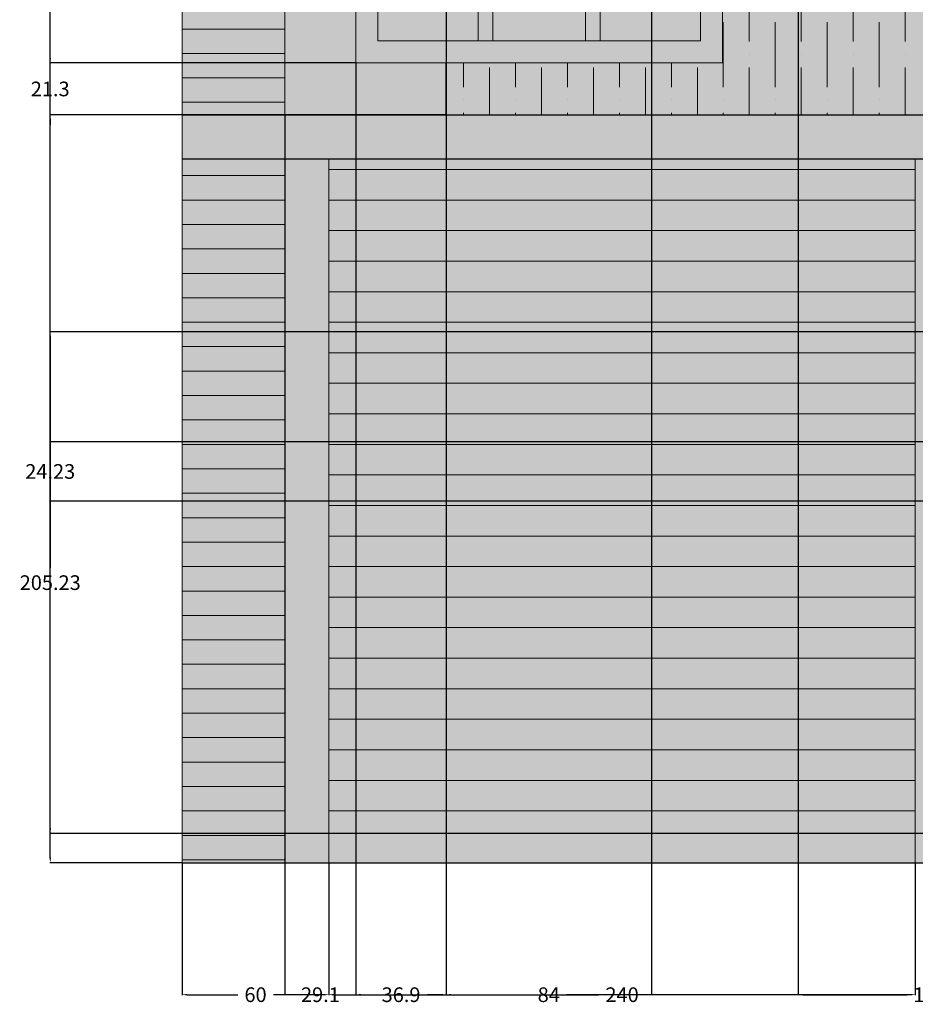
# Model space of a CAD drawing. Units: inches. Extents: x 180 to 1069, y 71 to 1267.
# Tile 1 of 8: x 180 to 546, y 71 to 474. Entities that reach past the tile are written whole.
import ezdxf

# ---------------------------------------------------------------- set-up
doc = ezdxf.new("R2010")
doc.units = ezdxf.units.IN
doc.header["$MEASUREMENT"] = 0
for name, color, linetype, lineweight in [('A-ANNO-DIMS', 2, 'Continuous', 18), ('A-ELEV-FRAM', 7, 'Continuous', 25), ('A-GLAZ', 7, 'Continuous', 18), ('A-WALL', 7, 'Continuous', 30), ('A-WALL-CLAD', 7, 'Continuous', 18), ('A-WALL-CLAD-JNTS-PATT', 18, 'Continuous', 13), ('A-WALL-CLAD-PATT', 26, 'Continuous', 13), ('A-WALL-SCRN-JNTS-PATT', 8, 'Continuous', 13)]:
    doc.layers.add(name, color=color, linetype=linetype, lineweight=lineweight)
for name, color, linetype, lineweight, true_color in [('A-DOOR-SHUT', 143, 'Continuous', 18, 0x7aafdf), ('A-DOOR-SHUT-PATT', 254, 'Continuous', 13, 0xb7d9eb), ('A-DOOR-SLAT-PATT', 143, 'Continuous', 13, 0x7aafdf), ('A-ELEV-BAND-PATT', 30, 'Continuous', 13, 0xf26722), ('A-ELEV-FRAM-PATT', 53, 'Continuous', 13, 0xefd648), ('A-ELEV-REVL-PATT', 9, 'Continuous', 13, 0xc7c8ca), ('A-ELEV-TRIM-PATT', 7, 'Continuous', 13, 0xffffff), ('A-WALL-SCRN-PATT', 251, 'Continuous', 13, 0x636466)]:
    doc.layers.add(name, color=color, linetype=linetype, lineweight=lineweight, true_color=true_color)
doc.styles.get("Standard").update_dxf_attribs({"font": 'arial.ttf'})
doc.dimstyles.get("Standard").update_dxf_attribs({"dimtxt": 6, "dimasz": 2, "dimexe": 0.18, "dimexo": 0.0625, "dimgap": 3, "dimtad": 0, "dimtih": 1, "dimtoh": 1, "dimdec": 0, "dimzin": 0, "dimdsep": 46, "dimlunit": 3, "dimtxsty": 'Standard', "dimcen": 0.09, "dimadec": 0, "dimazin": 0, "dimtfac": 1, "dimtdec": 0, "dimtofl": 0, "dimtmove": 0, "dimatfit": 3, "dimfxl": 1, "dimtolj": 1, "dimtzin": 0, "dimarcsym": 0})

# ---------------------------------------------------------------- blocks, each defined once
blk = doc.blocks.new('WIN-THREE-LIGHT')
for p, q in [((50, 9), (50, 51)), ((56, 9), (56, 51)), ((94, 9), (94, 51)), ((100, 9), (100, 51))]:
    blk.add_line(p, q)
for points in [[(0, 60), (150, 60), (150, 0), (0, 0)], [(9, 51), (141, 51), (141, 9), (9, 9)]]:
    blk.add_lwpolyline(points, close=True)
blk = doc.blocks.new('*D17')
at = {"layer": 'A-ANNO-DIMS', "color": 0, "lineweight": -2, "transparency": 16777216}
for p, q in [((246.02, 1208.82), (191.89, 1208.82)), ((192.07, 1206.82), (192.07, 674.88)), ((192.07, 130.82), (192.07, 662.75)), ((246.02, 128.82), (191.89, 128.82))]:
    blk.add_line(p, q, dxfattribs=at)
at = {"layer": 'A-ANNO-DIMS', "color": 0, "transparency": 16777216}
for points in [[(191.74, 1206.82), (192.41, 1206.82), (192.07, 1208.82)], [(191.74, 130.82), (192.41, 130.82), (192.07, 128.82)]]:
    blk.add_solid(points, dxfattribs=at)
at = {"layer": 'Defpoints', "color": 0, "transparency": 16777216}
for p in [(192.07, 1208.82), (246.09, 1208.82), (246.09, 128.82)]:
    blk.add_point(p, dxfattribs=at)
at = {"layer": 'A-ANNO-DIMS', "color": 0, "transparency": 16777216, "insert": (192.07, 668.82), "char_height": 6, "attachment_point": 5}
blk.add_mtext('\\A1;1080', dxfattribs=at)
blk = doc.blocks.new('*D28')
at = {"layer": 'A-ANNO-DIMS', "color": 0, "lineweight": -2, "transparency": 16777216}
for p, q in [((246.09, 128.75), (246.09, 74.62)), ((306.09, 128.75), (306.09, 74.62)), ((248.09, 74.8), (268.78, 74.8)), ((304.09, 74.8), (283.39, 74.8))]:
    blk.add_line(p, q, dxfattribs=at)
at = {"layer": 'A-ANNO-DIMS', "color": 0, "transparency": 16777216}
for points in [[(248.09, 75.14), (248.09, 74.47), (246.09, 74.8)], [(304.09, 75.14), (304.09, 74.47), (306.09, 74.8)]]:
    blk.add_solid(points, dxfattribs=at)
at = {"layer": 'Defpoints', "color": 0, "transparency": 16777216}
for p in [(246.09, 128.82), (306.09, 128.82), (306.09, 74.8)]:
    blk.add_point(p, dxfattribs=at)
at = {"layer": 'A-ANNO-DIMS', "color": 0, "transparency": 16777216, "insert": (276.09, 74.8), "char_height": 6, "attachment_point": 5}
blk.add_mtext('\\A1;60', dxfattribs=at)
blk = doc.blocks.new('*D29')
at = {"layer": 'A-ANNO-DIMS', "color": 0, "lineweight": -2, "transparency": 16777216}
for p, q in [((306.09, 128.75), (306.09, 74.62)), ((546.09, 128.75), (546.09, 74.62)), ((308.09, 74.8), (416.42, 74.8)), ((544.09, 74.8), (435.76, 74.8))]:
    blk.add_line(p, q, dxfattribs=at)
at = {"layer": 'A-ANNO-DIMS', "color": 0, "transparency": 16777216}
for points in [[(308.09, 75.14), (308.09, 74.47), (306.09, 74.8)], [(544.09, 75.14), (544.09, 74.47), (546.09, 74.8)]]:
    blk.add_solid(points, dxfattribs=at)
at = {"layer": 'Defpoints', "color": 0, "transparency": 16777216}
for p in [(306.09, 128.82), (546.09, 128.82), (546.09, 74.8)]:
    blk.add_point(p, dxfattribs=at)
at = {"layer": 'A-ANNO-DIMS', "color": 0, "transparency": 16777216, "insert": (426.09, 74.8), "char_height": 6, "attachment_point": 5}
blk.add_mtext('\\A1;240', dxfattribs=at)
blk = doc.blocks.new('*D39')
at = {"layer": 'A-ANNO-DIMS', "color": 0, "lineweight": -2, "transparency": 16777216}
for p, q in [((630.02, 346.05), (191.89, 346.05)), ((192.07, 344.05), (192.07, 249.5)), ((192.07, 142.82), (192.07, 237.37)), ((630.02, 140.82), (191.89, 140.82))]:
    blk.add_line(p, q, dxfattribs=at)
at = {"layer": 'A-ANNO-DIMS', "color": 0, "transparency": 16777216}
for points in [[(191.74, 344.05), (192.41, 344.05), (192.07, 346.05)], [(191.74, 142.82), (192.41, 142.82), (192.07, 140.82)]]:
    blk.add_solid(points, dxfattribs=at)
at = {"layer": 'Defpoints', "color": 0, "transparency": 16777216}
for p in [(192.07, 346.05), (630.09, 346.05), (630.09, 140.82)]:
    blk.add_point(p, dxfattribs=at)
at = {"layer": 'A-ANNO-DIMS', "color": 0, "transparency": 16777216, "insert": (192.07, 243.43), "char_height": 6, "attachment_point": 5}
blk.add_mtext('\\A1;205.23', dxfattribs=at)
blk = doc.blocks.new('*D43')
at = {"layer": 'A-ANNO-DIMS', "color": 0, "lineweight": -2, "transparency": 16777216}
for p, q in [((670.02, 301.05), (191.89, 301.05)), ((192.07, 299.05), (192.07, 295)), ((192.07, 278.82), (192.07, 282.87)), ((670.02, 276.82), (191.89, 276.82))]:
    blk.add_line(p, q, dxfattribs=at)
at = {"layer": 'A-ANNO-DIMS', "color": 0, "transparency": 16777216}
for points in [[(191.74, 299.05), (192.41, 299.05), (192.07, 301.05)], [(191.74, 278.82), (192.41, 278.82), (192.07, 276.82)]]:
    blk.add_solid(points, dxfattribs=at)
at = {"layer": 'Defpoints', "color": 0, "transparency": 16777216}
for p in [(670.09, 301.05), (192.07, 276.82), (670.09, 276.82)]:
    blk.add_point(p, dxfattribs=at)
at = {"layer": 'A-ANNO-DIMS', "color": 0, "transparency": 16777216, "insert": (192.07, 288.93), "char_height": 6, "attachment_point": 5}
blk.add_mtext('\\A1;24.23', dxfattribs=at)
blk = doc.blocks.new('*D50')
at = {"layer": 'A-ANNO-DIMS', "color": 0, "lineweight": -2, "transparency": 16777216}
for p, q in [((317.19, 456.06), (317.19, 74.62)), ((288.09, 434.75), (288.09, 74.62)), ((286.09, 74.8), (284.09, 74.8)), ((319.19, 74.8), (321.19, 74.8))]:
    blk.add_line(p, q, dxfattribs=at)
at = {"layer": 'A-ANNO-DIMS', "color": 0, "transparency": 16777216}
for points in [[(286.09, 75.14), (286.09, 74.47), (288.09, 74.8)], [(319.19, 75.14), (319.19, 74.47), (317.19, 74.8)]]:
    blk.add_solid(points, dxfattribs=at)
at = {"layer": 'Defpoints', "color": 0, "transparency": 16777216}
for p in [(317.19, 456.12), (288.09, 434.82), (317.19, 74.8)]:
    blk.add_point(p, dxfattribs=at)
at = {"layer": 'A-ANNO-DIMS', "color": 0, "transparency": 16777216, "insert": (302.64, 74.8), "char_height": 6, "attachment_point": 5}
blk.add_mtext('\\A1;29.1', dxfattribs=at)
blk = doc.blocks.new('*D51')
at = {"layer": 'A-ANNO-DIMS', "color": 0, "lineweight": -2, "transparency": 16777216}
for p, q in [((354.09, 624.01), (354.09, 74.62)), ((317.19, 456.06), (317.19, 74.62)), ((319.19, 74.8), (324.84, 74.8)), ((352.09, 74.8), (346.44, 74.8))]:
    blk.add_line(p, q, dxfattribs=at)
at = {"layer": 'A-ANNO-DIMS', "color": 0, "transparency": 16777216}
for points in [[(319.19, 75.14), (319.19, 74.47), (317.19, 74.8)], [(352.09, 75.14), (352.09, 74.47), (354.09, 74.8)]]:
    blk.add_solid(points, dxfattribs=at)
at = {"layer": 'Defpoints', "color": 0, "transparency": 16777216}
for p in [(354.09, 624.07), (317.19, 456.12), (354.09, 74.8)]:
    blk.add_point(p, dxfattribs=at)
at = {"layer": 'A-ANNO-DIMS', "color": 0, "transparency": 16777216, "insert": (335.64, 74.8), "char_height": 6, "attachment_point": 5}
blk.add_mtext('\\A1;36.9', dxfattribs=at)
blk = doc.blocks.new('*D52')
at = {"layer": 'A-ANNO-DIMS', "color": 0, "lineweight": -2, "transparency": 16777216}
for p, q in [((354.09, 624.01), (354.09, 74.62)), ((438.09, 624.01), (438.09, 74.62)), ((356.09, 74.8), (388.8, 74.8)), ((436.09, 74.8), (403.38, 74.8))]:
    blk.add_line(p, q, dxfattribs=at)
at = {"layer": 'A-ANNO-DIMS', "color": 0, "transparency": 16777216}
for points in [[(356.09, 75.14), (356.09, 74.47), (354.09, 74.8)], [(436.09, 75.14), (436.09, 74.47), (438.09, 74.8)]]:
    blk.add_solid(points, dxfattribs=at)
at = {"layer": 'Defpoints', "color": 0, "transparency": 16777216}
for p in [(354.09, 624.07), (438.09, 624.07), (438.09, 74.8)]:
    blk.add_point(p, dxfattribs=at)
at = {"layer": 'A-ANNO-DIMS', "color": 0, "transparency": 16777216, "insert": (396.09, 74.8), "char_height": 6, "attachment_point": 5}
blk.add_mtext('\\A1;84', dxfattribs=at)
blk = doc.blocks.new('*D56')
at = {"layer": 'A-ANNO-DIMS', "color": 0, "lineweight": -2, "transparency": 16777216}
for p, q in [((192.07, 458.12), (192.07, 460.12)), ((317.13, 456.12), (191.89, 456.12)), ((354.02, 434.82), (191.89, 434.82)), ((192.07, 432.82), (192.07, 430.82))]:
    blk.add_line(p, q, dxfattribs=at)
at = {"layer": 'A-ANNO-DIMS', "color": 0, "transparency": 16777216}
for points in [[(191.74, 458.12), (192.41, 458.12), (192.07, 456.12)], [(191.74, 432.82), (192.41, 432.82), (192.07, 434.82)]]:
    blk.add_solid(points, dxfattribs=at)
at = {"layer": 'Defpoints', "color": 0, "transparency": 16777216}
for p in [(192.07, 456.12), (317.19, 456.12), (354.09, 434.82)]:
    blk.add_point(p, dxfattribs=at)
at = {"layer": 'A-ANNO-DIMS', "color": 0, "transparency": 16777216, "insert": (192.07, 445.47), "char_height": 6, "attachment_point": 5}
blk.add_mtext('\\A1;21.3', dxfattribs=at)
blk = doc.blocks.new('*D58')
at = {"layer": 'A-ANNO-DIMS', "color": 0, "lineweight": -2, "transparency": 16777216}
for p, q in [((606.09, 1010.75), (606.09, 74.62)), ((498.09, 956.75), (498.09, 74.62)), ((500.09, 74.8), (542.74, 74.8)), ((604.09, 74.8), (561.44, 74.8))]:
    blk.add_line(p, q, dxfattribs=at)
at = {"layer": 'A-ANNO-DIMS', "color": 0, "transparency": 16777216}
for points in [[(500.09, 75.14), (500.09, 74.47), (498.09, 74.8)], [(604.09, 75.14), (604.09, 74.47), (606.09, 74.8)]]:
    blk.add_solid(points, dxfattribs=at)
at = {"layer": 'Defpoints', "color": 0, "transparency": 16777216}
for p in [(606.09, 1010.82), (498.09, 956.82), (606.09, 74.8)]:
    blk.add_point(p, dxfattribs=at)
at = {"layer": 'A-ANNO-DIMS', "color": 0, "transparency": 16777216, "insert": (552.09, 74.8), "char_height": 6, "attachment_point": 5}
blk.add_mtext('\\A1;108', dxfattribs=at)
blk = doc.blocks.new('*D60')
at = {"layer": 'A-ANNO-DIMS', "color": 0, "lineweight": -2, "transparency": 16777216}
for p, q in [((498.15, 488.82), (1056.28, 488.82)), ((1056.1, 486.82), (1056.1, 467.87)), ((1056.1, 436.82), (1056.1, 455.76)), ((606.15, 434.82), (1056.28, 434.82))]:
    blk.add_line(p, q, dxfattribs=at)
at = {"layer": 'A-ANNO-DIMS', "color": 0, "transparency": 16777216}
for points in [[(1055.77, 486.82), (1056.43, 486.82), (1056.1, 488.82)], [(1055.77, 436.82), (1056.43, 436.82), (1056.1, 434.82)]]:
    blk.add_solid(points, dxfattribs=at)
at = {"layer": 'Defpoints', "color": 0, "transparency": 16777216}
for p in [(498.09, 488.82), (606.09, 434.82), (1056.1, 434.82)]:
    blk.add_point(p, dxfattribs=at)
at = {"layer": 'A-ANNO-DIMS', "color": 0, "transparency": 16777216, "insert": (1056.1, 461.82), "char_height": 6, "attachment_point": 5}
blk.add_mtext('\\A1;54', dxfattribs=at)

msp = doc.modelspace()

# ---------------------------------------------------------------- hatches: boundary and pattern name
at = {"layer": 'A-DOOR-SHUT-PATT'}
h = msp.add_hatch(color=256, dxfattribs=at)
h.dxf.hatch_style = 1
h.paths.add_polyline_path([(546.0875, 416.8159), (306.0875, 416.8159), (306.0875, 140.8159), (546.0875, 140.8159)])
h.paths.add_polyline_path([(306.0875, 416.8159), (288.0875, 416.8159), (288.0875, 128.8159), (306.0875, 128.8159)])
h.paths.add_polyline_path([(546.0875, 140.8159), (306.0875, 140.8159), (306.0875, 128.8159), (546.0875, 128.8159)])
h.paths.add_polyline_path([(564.0875, 416.8159), (546.0875, 416.8159), (546.0875, 140.8159), (546.0875, 128.8159), (564.0875, 128.8159)])
at = {"layer": 'A-DOOR-SLAT-PATT'}
h = msp.add_hatch(dxfattribs=at)
h.set_pattern_fill('ANSI31', color=256, scale=100, angle=135)
h.paths.add_polyline_path([(546.0875, 416.8159), (306.0875, 416.8159), (306.0875, 140.8159), (546.0875, 140.8159)])
at = {"layer": 'A-ELEV-BAND-PATT'}
h = msp.add_hatch(color=256, dxfattribs=at)
h.dxf.hatch_style = 1
h.paths.add_polyline_path([(1002.0875, 1148.8159), (726.0875, 1148.8159), (726.0875, 1130.8159), (954.0875, 1130.8159), (954.0875, 947.2513), (978.0875, 947.2513), (978.0875, 1130.8159), (1002.0875, 1130.8159)])
h.paths.add_polyline_path([(654.0875, 1148.8159), (354.0875, 1148.8159), (354.0875, 1130.8159), (654.0875, 1130.8159)])
h.paths.add_polyline_path([(606.0875, 434.8159), (246.0875, 434.8159), (246.0875, 416.8159), (606.0875, 416.8159)])
h.paths.add_polyline_path([(978.0875, 845.8159), (726.0875, 845.8159), (726.0875, 791.8159), (978.0875, 791.8159)])
at = {"layer": 'A-ELEV-FRAM-PATT'}
h = msp.add_hatch(color=256, dxfattribs=at)
h.dxf.hatch_style = 1
h.paths.add_polyline_path([(354.0875, 1184.8159), (654.0875, 1184.8159), (654.0875, 974.8159), (726.0875, 974.8159), (726.0875, 1208.8159), (288.0875, 1208.8159), (288.0875, 897.6348), (304.7188, 897.6348), (304.7188, 883.4805), (288.0875, 883.4805), (288.0875, 866.8025), (304.7188, 866.8025), (304.7188, 852.6482), (288.0875, 852.6482), (288.0875, 835.9702), (304.7188, 835.9702), (304.7188, 821.8159), (288.0875, 821.8159), (288.0875, 805.1379), (304.7188, 805.1379), (304.7188, 790.9836), (288.0875, 790.9836), (288.0875, 774.3056), (304.7188, 774.3056), (304.7188, 760.1513), (288.0875, 760.1513), (288.0875, 743.4733), (304.7188, 743.4733), (304.7188, 729.319), (288.0875, 729.319), (288.0875, 434.8159), (354.0875, 434.8159), (354.0875, 456.1177), (317.1892, 456.1177), (317.1892, 516.1177), (354.0875, 516.1177), (354.0875, 924.0304), (317.1892, 924.0304), (317.1892, 984.0304), (354.0875, 984.0304)])
h.paths.add_polyline_path([(1002.0875, 869.8159), (702.0875, 869.8159), (702.0875, 791.8159), (726.0875, 791.8159), (726.0875, 845.8159), (978.0875, 845.8159), (978.0875, 581.8159), (726.0875, 581.8159), (726.0875, 647.8159), (702.0875, 647.8159), (702.0875, 557.8159), (1002.0875, 557.8159)])
h.paths.add_polyline_path([(906.0875, 1080.2003), (882.0875, 1080.2003), (882.0875, 1056.2003), (906.0875, 1056.2003)])
h.paths.add_polyline_path([(906.0875, 996.2003), (882.0875, 996.2003), (882.0875, 972.2003), (906.0875, 972.2003)])
h.paths.add_polyline_path([(636.5273, 869.8159), (612.5273, 869.8159), (612.5273, 845.8159), (636.5273, 845.8159)], flags=17)
h.paths.add_polyline_path([(682.6602, 869.8159), (658.6602, 869.8159), (658.6602, 845.8159), (682.6602, 845.8159)], flags=17)
h.paths.add_polyline_path([(636.5273, 581.8159), (612.5273, 581.8159), (612.5273, 557.8159), (636.5273, 557.8159)], flags=17)
h.paths.add_polyline_path([(682.6602, 581.8159), (658.6602, 581.8159), (658.6602, 557.8159), (682.6602, 557.8159)], flags=17)
h.paths.add_polyline_path([(942.0875, 358.0477), (918.0875, 358.0477), (918.0875, 128.8159), (942.0875, 128.8159)])
h.paths.add_polyline_path([(630.0875, 358.0477), (606.0875, 358.0477), (606.0875, 128.8159), (630.0875, 128.8159)])
at = {"layer": 'A-ELEV-REVL-PATT'}
h = msp.add_hatch(color=256, dxfattribs=at)
h.dxf.hatch_style = 1
h.paths.add_polyline_path([(426.0875, 680.0741), (354.0875, 680.0741), (354.0875, 672.0741), (426.0875, 672.0741)])
h.paths.add_polyline_path([(426.0875, 768.0741), (354.0875, 768.0741), (354.0875, 760.0741), (426.0875, 760.0741)])
h.paths.add_polyline_path([(417.1892, 507.1177), (411.1892, 507.1177), (411.1892, 465.1177), (417.1892, 465.1177)])
h.paths.add_polyline_path([(373.1892, 507.1177), (367.1892, 507.1177), (367.1892, 465.1177), (373.1892, 465.1177)])
h.paths.add_polyline_path([(373.1892, 975.0304), (367.1892, 975.0304), (367.1892, 933.0304), (373.1892, 933.0304)])
h.paths.add_polyline_path([(417.1892, 975.0304), (411.1892, 975.0304), (411.1892, 933.0304), (417.1892, 933.0304)])
at = {"layer": 'A-ELEV-TRIM-PATT'}
h = msp.add_hatch(color=256, dxfattribs=at)
h.dxf.hatch_style = 1
h.paths.add_polyline_path([(467.1892, 516.1177), (317.1892, 516.1177), (317.1892, 456.1177), (467.1892, 456.1177)])
h.paths.add_polyline_path([(458.1892, 507.1177), (458.1892, 465.1177), (326.1892, 465.1177), (326.1892, 507.1177)], flags=16)
h.paths.add_polyline_path([(354.0875, 816.0741), (354.0875, 804.0741), (426.0875, 804.0741), (426.0875, 636.0741), (354.0875, 636.0741), (354.0875, 624.0741), (438.0875, 624.0741), (438.0875, 816.0741)])
h.paths.add_polyline_path([(317.1892, 924.0304), (467.1892, 924.0304), (467.1892, 984.0304), (317.1892, 984.0304)])
h.paths.add_polyline_path([(326.1892, 933.0304), (326.1892, 975.0304), (458.1892, 975.0304), (458.1892, 933.0304)], flags=16)
h.paths.add_polyline_path([(304.7188, 897.6348), (262.2193, 897.6348), (262.2193, 883.4805), (304.7188, 883.4805)])
h.paths.add_polyline_path([(304.7188, 866.8025), (262.2193, 866.8025), (262.2193, 852.6482), (304.7188, 852.6482)])
h.paths.add_polyline_path([(304.7188, 835.9702), (262.2193, 835.9702), (262.2193, 821.8159), (304.7188, 821.8159)])
h.paths.add_polyline_path([(304.7188, 805.1379), (262.2193, 805.1379), (262.2193, 790.9836), (304.7188, 790.9836)])
h.paths.add_polyline_path([(304.7188, 774.3056), (262.2193, 774.3056), (262.2193, 760.1513), (304.7188, 760.1513)])
h.paths.add_polyline_path([(304.7188, 743.4733), (262.2193, 743.4733), (262.2193, 729.319), (304.7188, 729.319)])
h.paths.add_polyline_path([(600.0875, 370.0477), (600.0875, 358.0477), (636.0875, 358.0477), (636.0875, 370.0477)])
h.paths.add_polyline_path([(912.0875, 370.0477), (912.0875, 358.0477), (948.0875, 358.0477), (948.0875, 370.0477)])
at = {"layer": 'A-WALL-CLAD-JNTS-PATT'}
h = msp.add_hatch(dxfattribs=at)
h.set_pattern_fill('ANSI31', color=256, scale=80, angle=135)
h.paths.add_polyline_path([(288.0875, 416.8159), (246.0875, 416.8159), (246.0875, 128.8159), (288.0875, 128.8159)])
h.paths.add_polyline_path([(606.0875, 358.0477), (600.0875, 358.0477), (600.0875, 370.0477), (606.0875, 370.0477), (606.0875, 416.8159), (564.0875, 416.8159), (564.0875, 128.8159), (606.0875, 128.8159)])
h.paths.add_polyline_path([(288.0875, 729.319), (262.2193, 729.319), (262.2193, 743.4733), (288.0875, 743.4733), (288.0875, 760.1513), (262.2193, 760.1513), (262.2193, 774.3056), (288.0875, 774.3056), (288.0875, 790.9836), (262.2193, 790.9836), (262.2193, 805.1379), (288.0875, 805.1379), (288.0875, 821.8159), (262.2193, 821.8159), (262.2193, 835.9702), (288.0875, 835.9702), (288.0875, 852.6482), (262.2193, 852.6482), (262.2193, 866.8025), (288.0875, 866.8025), (288.0875, 883.4805), (262.2193, 883.4805), (262.2193, 897.6348), (288.0875, 897.6348), (288.0875, 1208.8159), (246.0875, 1208.8159), (246.0875, 434.8159), (288.0875, 434.8159)])
at = {"layer": 'A-WALL-CLAD-PATT'}
h = msp.add_hatch(color=256, dxfattribs=at)
h.dxf.hatch_style = 1
h.paths.add_polyline_path([(288.0875, 1208.8159), (246.0875, 1208.8159), (246.0875, 434.8159), (288.0875, 434.8159), (288.0875, 729.319), (262.2193, 729.319), (262.2193, 743.4733), (288.0875, 743.4733), (288.0875, 760.1513), (262.2193, 760.1513), (262.2193, 774.3056), (288.0875, 774.3056), (288.0875, 790.9836), (262.2193, 790.9836), (262.2193, 805.1379), (288.0875, 805.1379), (288.0875, 821.8159), (262.2193, 821.8159), (262.2193, 835.9702), (288.0875, 835.9702), (288.0875, 852.6482), (262.2193, 852.6482), (262.2193, 866.8025), (288.0875, 866.8025), (288.0875, 883.4805), (262.2193, 883.4805), (262.2193, 897.6348), (288.0875, 897.6348)])
h.paths.add_polyline_path([(288.0875, 416.8159), (246.0875, 416.8159), (246.0875, 128.8159), (288.0875, 128.8159)])
at = {"layer": 'A-WALL-SCRN-JNTS-PATT'}
h = msp.add_hatch(dxfattribs=at)
h.set_pattern_fill('ANSI36', color=256, scale=85, angle=45)
h.paths.add_polyline_path([(606.0875, 938.8159), (798.0875, 938.8159), (798.0875, 869.8159), (834.0875, 869.8159), (834.0875, 974.8159), (606.0875, 974.8159), (606.0875, 1010.8159), (354.0875, 1010.8159), (354.0875, 984.0304), (467.1892, 984.0304), (467.1892, 956.8159), (498.0875, 956.8159), (498.0875, 488.8159), (467.1892, 488.8159), (467.1892, 456.1177), (354.0875, 456.1177), (354.0875, 434.8159), (606.0875, 434.8159), (606.0875, 473.8159), (834.0875, 473.8159), (834.0875, 557.8159), (798.0875, 557.8159), (798.0875, 509.8159), (606.0875, 509.8159)])
at = {"layer": 'A-WALL-SCRN-PATT'}
h = msp.add_hatch(color=256, dxfattribs=at)
h.dxf.hatch_style = 1
h.paths.add_polyline_path([(606.0875, 938.8159), (798.0875, 938.8159), (798.0875, 869.8159), (834.0875, 869.8159), (834.0875, 974.8159), (606.0875, 974.8159), (606.0875, 1010.8159), (354.0875, 1010.8159), (354.0875, 984.0304), (467.1892, 984.0304), (467.1892, 956.8159), (498.0875, 956.8159), (498.0875, 488.8159), (467.1892, 488.8159), (467.1892, 456.1177), (354.0875, 456.1177), (354.0875, 434.8159), (606.0875, 434.8159), (606.0875, 473.8159), (834.0875, 473.8159), (834.0875, 557.8159), (798.0875, 557.8159), (798.0875, 509.8159), (606.0875, 509.8159)])
h.paths.add_polyline_path([(367.1892, 507.1177), (326.1892, 507.1177), (326.1892, 465.1177), (367.1892, 465.1177)])
h.paths.add_polyline_path([(411.1892, 507.1177), (373.1892, 507.1177), (373.1892, 465.1177), (411.1892, 465.1177)], flags=17)
h.paths.add_polyline_path([(458.1892, 507.1177), (417.1892, 507.1177), (417.1892, 465.1177), (458.1892, 465.1177)], flags=17)
h.paths.add_polyline_path([(426.0875, 672.0741), (354.0875, 672.0741), (354.0875, 636.0741), (426.0875, 636.0741)], flags=17)
h.paths.add_polyline_path([(426.0875, 760.0741), (354.0875, 760.0741), (354.0875, 680.0741), (426.0875, 680.0741)], flags=17)
h.paths.add_polyline_path([(426.0875, 804.0741), (354.0875, 804.0741), (354.0875, 768.0741), (426.0875, 768.0741)], flags=17)
h.paths.add_polyline_path([(367.1892, 975.0304), (326.1892, 975.0304), (326.1892, 933.0304), (367.1892, 933.0304)])
h.paths.add_polyline_path([(411.1892, 975.0304), (373.1892, 975.0304), (373.1892, 933.0304), (411.1892, 933.0304)], flags=17)
h.paths.add_polyline_path([(458.1892, 975.0304), (417.1892, 975.0304), (417.1892, 933.0304), (458.1892, 933.0304)], flags=17)

# ---------------------------------------------------------------- linework, layer by layer
at = {"layer": 'A-DOOR-SHUT'}
for p, q in [((306.0875, 128.8159), (306.0875, 416.8159)), ((546.0875, 416.8159), (546.0875, 128.8159)), ((306.0875, 140.8159), (546.0875, 140.8159))]:
    msp.add_line(p, q, dxfattribs=at)
at = {"layer": 'A-ELEV-FRAM'}
for p, q in [((354.0875, 434.8159), (354.0875, 456.1177)), ((246.0875, 434.8159), (606.0875, 434.8159)), ((246.0875, 416.8159), (606.0875, 416.8159))]:
    msp.add_line(p, q, dxfattribs=at)
at = {"layer": 'A-WALL'}
msp.add_line((246.0875, 128.8159), (978.0875, 128.8159), dxfattribs=at)
at = {"layer": 'A-WALL-CLAD'}
for p, q in [((246.0875, 128.8159), (246.0875, 1208.8159)), ((288.0875, 434.8159), (288.0875, 729.319)), ((288.0875, 128.8159), (288.0875, 416.8159))]:
    msp.add_line(p, q, dxfattribs=at)

# ---------------------------------------------------------------- block references
at = {"layer": 'A-GLAZ'}
msp.add_blockref('WIN-THREE-LIGHT', (317.1892, 456.1177), dxfattribs=at)

# ---------------------------------------------------------------- dimensions: what is measured, and where the dimension line sits
at = {"layer": 'A-ANNO-DIMS'}
for base, p1, p2, override, picture, middle in [((192.074, 1208.8159), (246.0875, 128.8159), (246.0875, 1208.8159), {"dimdec": 0, "dimlfac": 1, "dimrnd": 0, "dimzin": 0, "dimdsep": 46, "dimlunit": 2}, '*D17', (192.074, 668.8159)), ((1056.101, 434.8159), (498.0875, 488.8159), (606.0875, 434.8159), {"dimdec": 0, "dimlfac": 1, "dimrnd": 0, "dimzin": 0, "dimdsep": 46, "dimlunit": 2}, '*D60', (1056.101, 461.8159)), ((192.074, 456.1177), (354.0875, 434.8159), (317.1892, 456.1177), {"dimdec": 1, "dimlfac": 1, "dimrnd": 0, "dimzin": 0, "dimdsep": 46, "dimlunit": 2}, '*D56', (192.074, 445.4668)), ((192.074, 346.0477), (630.0875, 140.8159), (630.0875, 346.0477), {"dimdec": 2, "dimlfac": 1, "dimrnd": 0, "dimzin": 0, "dimdsep": 46, "dimlunit": 2}, '*D39', (192.074, 243.4318)), ((192.074, 276.8159), (670.0875, 301.0477), (670.0875, 276.8159), {"dimdec": 2, "dimlfac": 1, "dimrnd": 0, "dimzin": 0, "dimdsep": 46, "dimlunit": 2}, '*D43', (192.074, 288.9318))]:
    dim = msp.add_linear_dim(base=base, p1=p1, p2=p2, angle=90, dimstyle='Standard', override=override, dxfattribs=at)
    dim.commit()
    dim.dimension.update_dxf_attribs({"geometry": picture, "text_midpoint": middle})
for base, p1, p2, override, picture, middle in [((606.0875, 74.8024), (498.0875, 956.8159), (606.0875, 1010.8159), {"dimdec": 0, "dimlfac": 1, "dimrnd": 0, "dimzin": 0, "dimdsep": 46, "dimlunit": 2}, '*D58', (552.0875, 74.8024)), ((354.0875, 74.8024), (317.1892, 456.1177), (354.0875, 624.0741), {"dimdec": 1, "dimlfac": 1, "dimrnd": 0, "dimzin": 0, "dimdsep": 46, "dimlunit": 2}, '*D51', (335.6383, 74.8024)), ((438.0875, 74.8024), (354.0875, 624.0741), (438.0875, 624.0741), {"dimdec": 0, "dimlfac": 1, "dimrnd": 0, "dimzin": 0, "dimdsep": 46, "dimlunit": 2}, '*D52', (396.0875, 74.8024)), ((317.1892, 74.8024), (288.0875, 434.8159), (317.1892, 456.1177), {"dimdec": 1, "dimlfac": 1, "dimrnd": 0, "dimzin": 0, "dimdsep": 46, "dimlunit": 2}, '*D50', (302.6383, 74.8024)), ((306.0875, 74.8024), (246.0875, 128.8159), (306.0875, 128.8159), {"dimdec": 0, "dimlfac": 1, "dimrnd": 0, "dimzin": 0, "dimdsep": 46, "dimlunit": 2}, '*D28', (276.0875, 74.8024)), ((546.0875, 74.8024), (306.0875, 128.8159), (546.0875, 128.8159), {"dimdec": 0, "dimlfac": 1, "dimrnd": 0, "dimzin": 0, "dimdsep": 46, "dimlunit": 2}, '*D29', (426.0875, 74.8024))]:
    dim = msp.add_linear_dim(base=base, p1=p1, p2=p2, dimstyle='Standard', override=override, dxfattribs=at)
    dim.commit()
    dim.dimension.update_dxf_attribs({"geometry": picture, "text_midpoint": middle})

doc.saveas('drawing.dxf')
